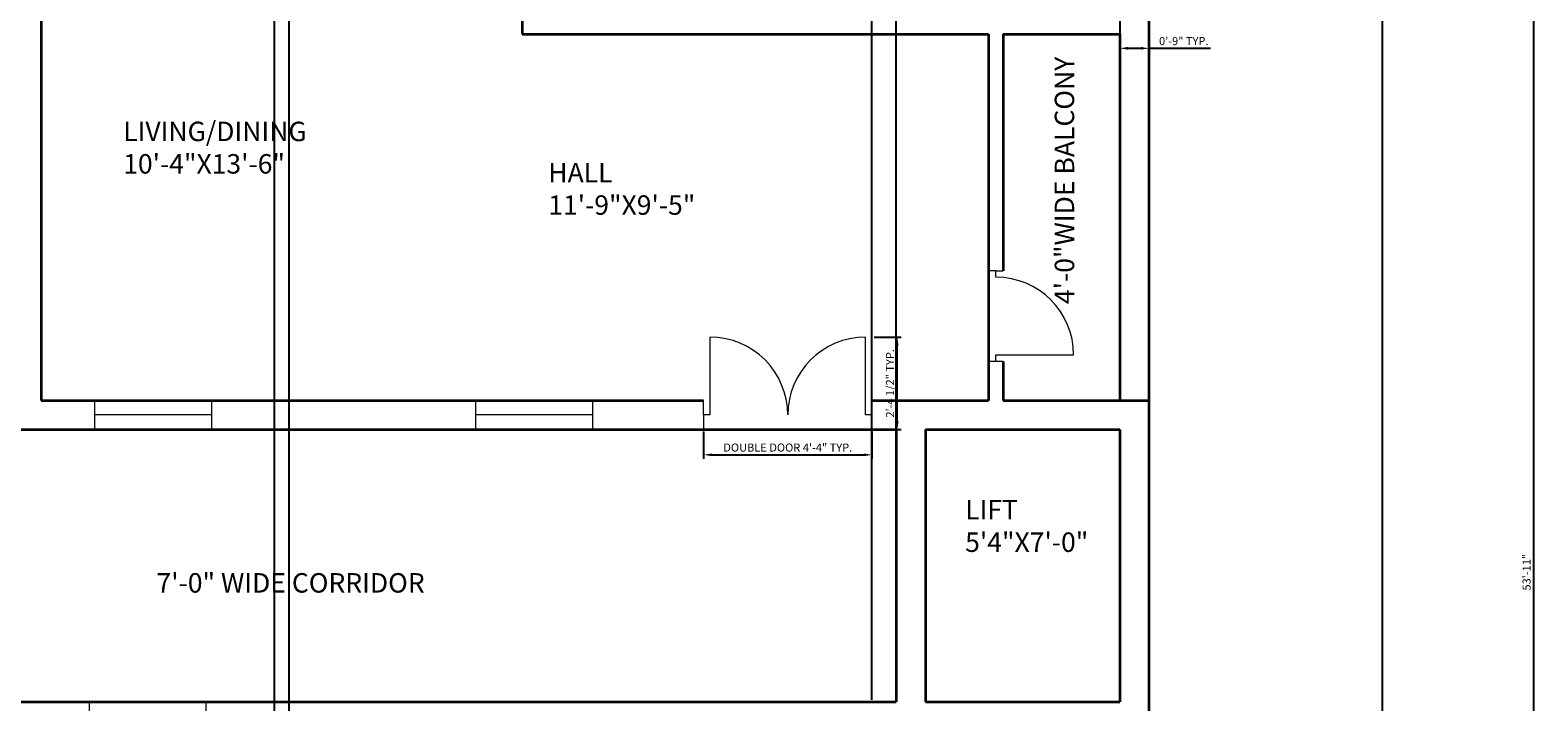
# Model space of a CAD drawing. Units: inches. Extents: x 3257 to 4085, y -12 to 956.
# Tile 5 of 6: x 3619 to 4085, y 441 to 648. Entities that reach past the tile are written whole.
import ezdxf

# ---------------------------------------------------------------- set-up
doc = ezdxf.new("R2010")
doc.units = ezdxf.units.IN
for name, color, linetype, lineweight in [('A-ANNO-DIMS', 2, 'Continuous', 18), ('A-AREA-IDEN', 7, 'Continuous', 18), ('A-DOOR', 3, 'Continuous', 18), ('A-GLAZ', 4, 'Continuous', 18), ('A-WALL', 7, 'Continuous', 35), ('C-PROP', 6, 'Continuous', 25)]:
    doc.layers.add(name, color=color, linetype=linetype, lineweight=lineweight)
doc.styles.get("Standard").update_dxf_attribs({"font": 'arial.ttf'})
doc.dimstyles.new('ISO-25', dxfattribs={"dimtxt": 2.5, "dimasz": 2.5, "dimexe": 1.25, "dimexo": 0.625, "dimtad": 1, "dimdec": 0, "dimlunit": 3, "dimtxsty": 'Standard', "dimcen": 2.5, "dimadec": 0, "dimazin": 0, "dimtfac": 1, "dimtdec": 0, "dimtmove": 0, "dimatfit": 3, "dimfxl": 1, "dimarcsym": 0})

# ---------------------------------------------------------------- blocks, each defined once
blk = doc.blocks.new('DOOR-SGL-24IN')
for p, q in [((2.25, 28), (0, 28)), ((2.25, 26), (2.25, 28)), ((2.25, 28), (4.5, 28)), ((2.25, 0), (2.25, 2)), ((2.25, 2), (26.25, 2)), ((4.5, 0), (0, 0))]:
    blk.add_line(p, q)
blk.add_arc((2.25, 2), 24, 0, 90)
blk = doc.blocks.new('WIN-36IN')
for p, q in [((0, 9), (36, 9)), ((0, 0), (0, 9)), ((36, 9), (36, 0)), ((0, 4.5), (36, 4.5)), ((36, 0), (0, 0))]:
    blk.add_line(p, q)
blk = doc.blocks.new('DOOR-DBL-2X24IN')
for p, q in [((2, 4.5), (2, 28.5)), ((50, 4.5), (50, 28.5)), ((0, 4.5), (0, 9)), ((52, 9), (52, 0)), ((2, 4.5), (0, 4.5)), ((0, 4.5), (0, 0)), ((52, 4.5), (50, 4.5))]:
    blk.add_line(p, q)
for centre, start, end in [((2, 4.5), 0, 90), ((50, 4.5), 90, 180)]:
    blk.add_arc(centre, 24, start, end)
blk = doc.blocks.new('*D10')
at = {"layer": 'A-ANNO-DIMS', "color": 0, "lineweight": -2, "transparency": 16777216}
for p, q in [((3826.97, 523.88), (3826.97, 515.45)), ((3878.97, 523.88), (3878.97, 515.45)), ((3829.47, 516.7), (3876.47, 516.7))]:
    blk.add_line(p, q, dxfattribs=at)
at = {"layer": 'A-ANNO-DIMS', "color": 0, "transparency": 16777216}
for points in [[(3829.47, 517.12), (3829.47, 516.29), (3826.97, 516.7)], [(3876.47, 517.12), (3876.47, 516.29), (3878.97, 516.7)]]:
    blk.add_solid(points, dxfattribs=at)
at = {"layer": 'Defpoints', "color": 0, "transparency": 16777216}
for p in [(3826.97, 524.5), (3878.97, 524.5), (3878.97, 516.7)]:
    blk.add_point(p, dxfattribs=at)
at = {"layer": 'A-ANNO-DIMS', "color": 0, "transparency": 16777216, "insert": (3852.97, 518.62), "char_height": 2.5, "attachment_point": 5}
blk.add_mtext('DOUBLE DOOR 4\'-4" TYP.', dxfattribs=at)
blk = doc.blocks.new('*D11')
at = {"layer": 'A-ANNO-DIMS', "color": 0, "lineweight": -2, "transparency": 16777216}
for p, q in [((3879.59, 553), (3888.02, 553)), ((3886.77, 527), (3886.77, 550.5)), ((3879.59, 524.5), (3888.02, 524.5))]:
    blk.add_line(p, q, dxfattribs=at)
at = {"layer": 'A-ANNO-DIMS', "color": 0, "transparency": 16777216}
for points in [[(3886.35, 550.5), (3887.18, 550.5), (3886.77, 553)], [(3886.35, 527), (3887.18, 527), (3886.77, 524.5)]]:
    blk.add_solid(points, dxfattribs=at)
at = {"layer": 'Defpoints', "color": 0, "transparency": 16777216}
for p in [(3878.97, 553), (3886.77, 553), (3878.97, 524.5)]:
    blk.add_point(p, dxfattribs=at)
at = {"layer": 'A-ANNO-DIMS', "color": 0, "transparency": 16777216, "insert": (3884.85, 538.75), "char_height": 2.5, "attachment_point": 5, "rotation": 90}
blk.add_mtext('2\'-4 1/2" TYP.', dxfattribs=at)
blk = doc.blocks.new('*D17')
at = {"layer": 'A-ANNO-DIMS', "color": 0, "lineweight": -2, "transparency": 16777216}
for p, q in [((3955.47, 650.49), (3955.47, 640.86)), ((3964.47, 650.49), (3964.47, 640.86)), ((3957.97, 642.11), (3961.97, 642.11)), ((3964.47, 642.11), (3983.46, 642.11))]:
    blk.add_line(p, q, dxfattribs=at)
at = {"layer": 'A-ANNO-DIMS', "color": 0, "transparency": 16777216}
for points in [[(3957.97, 642.53), (3957.97, 641.69), (3955.47, 642.11)], [(3961.97, 642.53), (3961.97, 641.69), (3964.47, 642.11)]]:
    blk.add_solid(points, dxfattribs=at)
at = {"layer": 'Defpoints', "color": 0, "transparency": 16777216}
for p in [(3955.47, 651.11), (3964.47, 651.11), (3964.47, 642.11)]:
    blk.add_point(p, dxfattribs=at)
at = {"layer": 'A-ANNO-DIMS', "color": 0, "transparency": 16777216, "insert": (3975.21, 644.01), "char_height": 2.5, "attachment_point": 5}
blk.add_mtext('0\'-9" TYP.', dxfattribs=at)
blk = doc.blocks.new('*D19')
at = {"layer": 'A-ANNO-DIMS', "color": 0, "lineweight": -2, "transparency": 16777216}
for p, q in [((3965.09, 804), (4084.52, 804)), ((4083.27, 159.5), (4083.27, 801.5)), ((3965.09, 157), (4084.52, 157))]:
    blk.add_line(p, q, dxfattribs=at)
at = {"layer": 'A-ANNO-DIMS', "color": 0, "transparency": 16777216}
for points in [[(4082.85, 801.5), (4083.68, 801.5), (4083.27, 804)], [(4082.85, 159.5), (4083.68, 159.5), (4083.27, 157)]]:
    blk.add_solid(points, dxfattribs=at)
at = {"layer": 'Defpoints', "color": 0, "transparency": 16777216}
for p in [(3964.47, 804), (4083.27, 804), (3964.47, 157)]:
    blk.add_point(p, dxfattribs=at)
at = {"layer": 'A-ANNO-DIMS', "color": 0, "transparency": 16777216, "insert": (4081.37, 480.5), "char_height": 2.5, "attachment_point": 5, "rotation": 90}
blk.add_mtext('53\'-11"', dxfattribs=at)
blk = doc.blocks.new('*D25')
at = {"layer": 'A-ANNO-DIMS', "color": 0, "lineweight": -2, "transparency": 16777216}
for p, q in [((3878.97, 441.13), (3878.97, 924.05)), ((3881.47, 922.8), (3883.97, 922.8)), ((3886.47, 441.13), (3886.47, 924.05)), ((3886.47, 922.8), (3902.69, 922.8))]:
    blk.add_line(p, q, dxfattribs=at)
at = {"layer": 'A-ANNO-DIMS', "color": 0, "transparency": 16777216}
for points in [[(3881.47, 923.22), (3881.47, 922.39), (3878.97, 922.8)], [(3883.97, 923.22), (3883.97, 922.39), (3886.47, 922.8)]]:
    blk.add_solid(points, dxfattribs=at)
at = {"layer": 'Defpoints', "color": 0, "transparency": 16777216}
for p in [(3886.47, 922.8), (3878.97, 440.5), (3886.47, 440.5)]:
    blk.add_point(p, dxfattribs=at)
at = {"layer": 'A-ANNO-DIMS', "color": 0, "transparency": 16777216, "insert": (3895.83, 924.72), "char_height": 2.5, "attachment_point": 5}
blk.add_mtext('0\'-7 1/2"', dxfattribs=at)
blk = doc.blocks.new('*D26')
at = {"layer": 'A-ANNO-DIMS', "color": 0, "lineweight": -2, "transparency": 16777216}
for p, q in [((3694.47, 710.38), (3694.47, -11.05)), ((3698.97, 710.38), (3698.97, -11.05)), ((3691.97, -9.8), (3689.47, -9.8)), ((3694.47, -9.8), (3698.97, -9.8)), ((3701.47, -9.8), (3717.69, -9.8))]:
    blk.add_line(p, q, dxfattribs=at)
at = {"layer": 'A-ANNO-DIMS', "color": 0, "transparency": 16777216}
for points in [[(3691.97, -9.38), (3691.97, -10.21), (3694.47, -9.8)], [(3701.47, -9.38), (3701.47, -10.21), (3698.97, -9.8)]]:
    blk.add_solid(points, dxfattribs=at)
at = {"layer": 'Defpoints', "color": 0, "transparency": 16777216}
for p in [(3694.47, 711), (3698.97, 711), (3698.97, -9.8)]:
    blk.add_point(p, dxfattribs=at)
at = {"layer": 'A-ANNO-DIMS', "color": 0, "transparency": 16777216, "insert": (3710.83, -7.88), "char_height": 2.5, "attachment_point": 5}
blk.add_mtext('0\'-4 1/2"', dxfattribs=at)

msp = doc.modelspace()

# ---------------------------------------------------------------- linework, layer by layer
at = {"layer": 'A-WALL'}
for p, q in [((3964.47, 685), (3964.47, 157)), ((3622.47, 657), (3622.47, 533.5)), ((3770.97, 657), (3770.97, 646.5)), ((3770.97, 646.5), (3914.97, 646.5)), ((3914.97, 646.5), (3914.97, 533.5)), ((3919.47, 646.5), (3919.47, 573.5)), ((3919.47, 646.5), (3955.47, 646.5)), ((3955.47, 646.5), (3955.47, 533.5)), ((3919.47, 545.5), (3919.47, 533.5)), ((3622.47, 533.5), (3826.97, 533.5)), ((3878.97, 533.5), (3914.97, 533.5)), ((3919.47, 533.5), (3964.47, 533.5)), ((3411.97, 524.5), (3886.47, 524.5)), ((3886.47, 524.5), (3886.47, 440.5)), ((3895.47, 524.5), (3895.47, 440.5)), ((3895.47, 524.5), (3955.47, 524.5)), ((3955.47, 524.5), (3955.47, 440.5)), ((3411.97, 440.5), (3886.47, 440.5)), ((3895.47, 440.5), (3955.47, 440.5))]:
    msp.add_line(p, q, dxfattribs=at)
at = {"layer": 'C-PROP'}
msp.add_line((4036.47, 685), (4036.47, 37), dxfattribs=at)

# ---------------------------------------------------------------- block references
at = {"layer": 'A-DOOR'}
for name, p in [('DOOR-SGL-24IN', (3914.97, 545.5)), ('DOOR-DBL-2X24IN', (3826.97, 524.5))]:
    msp.add_blockref(name, p, dxfattribs=at)
at = {"layer": 'A-GLAZ', "rotation": 180}
for p in [(3675.07, 533.5), (3792.66, 533.5), (3673.37, 440.5)]:
    msp.add_blockref('WIN-36IN', p, dxfattribs=at)

# ---------------------------------------------------------------- texts
at = {"layer": 'A-AREA-IDEN', "insert": (3935.38, 563.2), "char_height": 6, "attachment_point": 1, "rotation": 90}
msp.add_mtext('4\'-0"WIDE BALCONY', dxfattribs=at)
at = {"layer": 'A-AREA-IDEN', "insert": (3647.82, 619.47), "char_height": 6, "attachment_point": 1}
msp.add_mtext_dynamic_manual_height_columns('LIVING/DINING\\P10\'-4"X13\'-6"', width=30.2379, gutter_width=12.5, heights=[0], dxfattribs=at)
at = {"layer": 'A-AREA-IDEN', "char_height": 6, "attachment_point": 1}
for s, insert in [('HALL\\P11\'-9"X9\'-5" ', (3779.04, 606.75)), ('LIFT\\P5\'4"X7\'-0"', (3907.73, 502.75)), ('7\'-0" WIDE CORRIDOR', (3658.1, 480.2))]:
    msp.add_mtext(s, dxfattribs=dict(at, insert=insert))

# ---------------------------------------------------------------- dimensions: what is measured, and where the dimension line sits
at = {"layer": 'A-ANNO-DIMS'}
for base, p1, p2, picture, middle in [((3886.47, 922.8), (3878.97, 440.5), (3886.47, 440.5), '*D25', (3895.83, 924.72)), ((3698.97, -9.8), (3694.47, 711), (3698.97, 711), '*D26', (3710.83, -7.88))]:
    dim = msp.add_linear_dim(base=base, p1=p1, p2=p2, dimstyle='ISO-25', override={"dimdec": 1, "dimlfac": 1, "dimrnd": 0, "dimzin": 1, "dimdsep": 46, "dimlunit": 4, "dimfrac": 2}, dxfattribs=at)
    dim.commit()
    dim.dimension.update_dxf_attribs({"geometry": picture, "text_midpoint": middle})
dim = msp.add_linear_dim(base=(4083.27, 804), p1=(3964.47, 157), p2=(3964.47, 804), angle=90, dimstyle='ISO-25', override={"dimdec": 1, "dimlfac": 1, "dimrnd": 0, "dimzin": 1, "dimdsep": 46, "dimlunit": 4, "dimfrac": 2}, dxfattribs=at)
dim.commit()
dim.dimension.update_dxf_attribs({"geometry": '*D19', "text_midpoint": (4081.37, 480.5)})
for base, p1, p2, text, picture, middle in [((3964.47, 642.11), (3955.47, 651.11), (3964.47, 651.11), '<> TYP.', '*D17', (3975.21, 644.01)), ((3878.97, 516.7), (3826.97, 524.5), (3878.97, 524.5), 'DOUBLE DOOR <> TYP.', '*D10', (3852.97, 518.62))]:
    dim = msp.add_linear_dim(base=base, p1=p1, p2=p2, text=text, dimstyle='ISO-25', override={"dimdec": 1, "dimlfac": 1, "dimrnd": 0, "dimzin": 1, "dimdsep": 46, "dimlunit": 4, "dimfrac": 2}, dxfattribs=at)
    dim.commit()
    dim.dimension.update_dxf_attribs({"geometry": picture, "text_midpoint": middle})
dim = msp.add_linear_dim(base=(3886.77, 553), p1=(3878.97, 524.5), p2=(3878.97, 553), angle=90, text='<> TYP.', dimstyle='ISO-25', override={"dimdec": 1, "dimlfac": 1, "dimrnd": 0, "dimzin": 1, "dimdsep": 46, "dimlunit": 4, "dimfrac": 2}, dxfattribs=at)
dim.commit()
dim.dimension.update_dxf_attribs({"geometry": '*D11', "text_midpoint": (3884.85, 538.75)})

doc.saveas('drawing.dxf')
